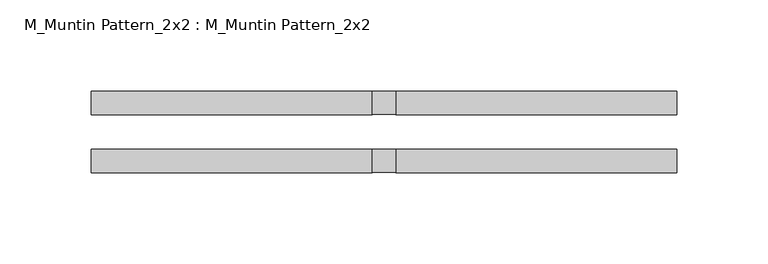
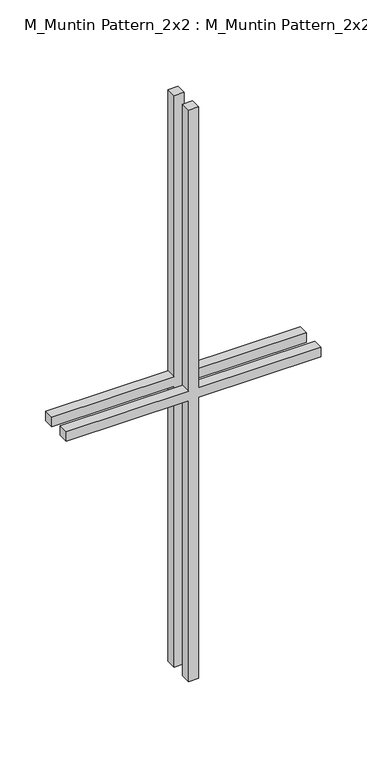
"""IFC4 building model written with IfcOpenShell, lengths in millimetres: proxy geometry, M_Muntin Pattern_2x2 : M_Muntin Pattern_2x2."""

from ifc_helpers import new_model, si_unit, frame, origin, place, context, project, spatial, polyline, outline, extrude, source, transform, mapped, element, save


def m_muntin_pattern_2x2_m_muntin_pattern_2x2_55460d9e(model_context):
    return source(origin(), model_context, "Body", "SweptSolid", [
        extrude(outline(polyline([(386.5, -6.35), (386.5, -160.3375), (373.8, -160.3375), (373.8, -6.35), (0.0, -6.35), (0.0, 6.35), (373.8, 6.35), (373.8, 160.3375), (386.5, 160.3375), (386.5, 6.35), (760.3, 6.35), (760.3, -6.35), (386.5, -6.35)])), frame((0.0, 9.525, 0.0), z_axis=(0.0, 1.0, 0.0), x_axis=(0.0, 0.0, 1.0)), (0.0, 0.0, 1.0), 12.7),
        extrude(outline(polyline([(386.5, -6.35), (386.5, -160.3375), (373.8, -160.3375), (373.8, -6.35), (0.0, -6.35), (0.0, 6.35), (373.8, 6.35), (373.8, 160.3375), (386.5, 160.3375), (386.5, 6.35), (760.3, 6.35), (760.3, -6.35), (386.5, -6.35)])), frame((0.0, -22.225, 0.0), z_axis=(0.0, 1.0, 0.0), x_axis=(0.0, 0.0, 1.0)), (0.0, 0.0, 1.0), 12.7),
    ])


if __name__ == "__main__":
    model = new_model("IFC4")
    model_context = context("Model", 3, world=origin())
    ifc_project = project(units=[si_unit("LENGTHUNIT", "METRE", prefix="MILLI")], contexts=[model_context])
    site = spatial("IfcSite", under=ifc_project)
    building = spatial("IfcBuilding", under=site)
    placement = place(None, origin())
    m_muntin_pattern_2x2_m_muntin_pattern_2x2_shape = m_muntin_pattern_2x2_m_muntin_pattern_2x2_55460d9e(model_context)
    element("IfcBuildingElementProxy", 1, Name="M_Muntin Pattern_2x2 : M_Muntin Pattern_2x2", ObjectType="M_Muntin Pattern_2x2 : M_Muntin Pattern_2x2", at=placement, inside=building, context=model_context, shape_type="MappedRepresentation", body=[
        mapped(m_muntin_pattern_2x2_m_muntin_pattern_2x2_shape, transform((0.0, 0.0, 0.0), x_axis=(1.0, 0.0, 0.0), y_axis=(0.0, 1.0, 0.0), z_axis=(0.0, 0.0, 1.0))),
    ])
    save(model, "model.ifc")

# Revit data of these elements
# Type "M_Muntin Pattern_2x2 : M_Muntin Pattern_2x2"
#   Width [instance default] = 3' - 11.24409"
#   Thickness = 0' - 0 1/2"
#   Height [instance default] = 3' - 11.24409"
#   Distance = 0' - 0 3/4"
#   Interior Material [instance default] = none
#   Exterior Material [instance default] = none
#   Default Elevation = 0
# Element 1 (IfcBuildingElementProxy, "M_Muntin Pattern_2x2 : M_Muntin Pattern_2x2")
#   Width = 1' - 0 5/8"
#   Height = 2' - 5.93307"
#   Interior Material = Wood - Stained
#   Exterior Material = Clad - White
#   Materials on its faces: "Clad - White", "Wood - Stained"
# Materials
#   "Clad - White": class "Wood", colour RGB 242 242 238, transparency 0, Cost = 0
#   "Wood - Stained": class "Wood", colour RGB 227 170 128, transparency 0, Cost = 0
